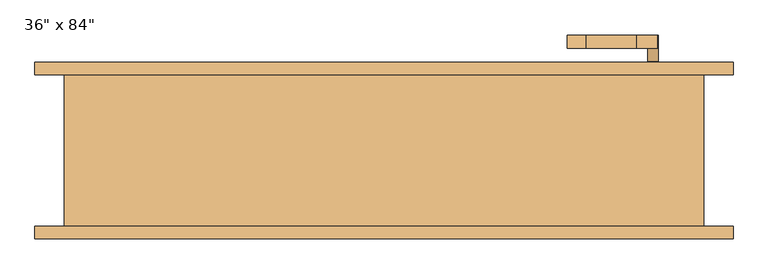
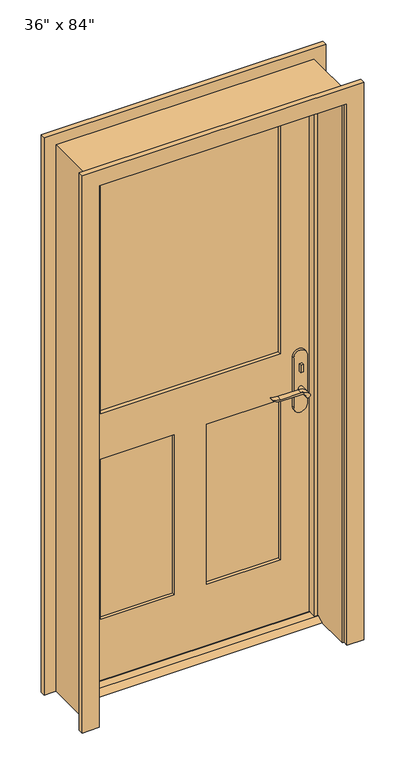
"""IFC4 building model written with IfcOpenShell, lengths in millimetres: door geometry."""

from ifc_helpers import new_model, si_unit, point, frame, frame_2d, origin, place, context, project, spatial, polyline, circle_curve, trimmed, segment, composite_curve, outline, extrude, faceted_brep, source, transform, mapped, element, save


def door_16625766(model_context):
    return source(origin(), model_context, "Body", "SolidModel", [
        extrude(outline(polyline([(38.1, 12.7), (73.025, 12.7), (98.425, 0.0), (12.7, 0.0), (38.1, 12.7)])), frame((-457.2, 0.0, 0.0), z_axis=(1.0, 0.0, 0.0), x_axis=(0.0, 1.0, 0.0)), (0.0, 0.0, 1.0), 914.4),
        extrude(outline(polyline([(411.4, 56.2), (401.4, 56.2), (401.4, 66.2), (411.4, 66.2), (411.4, 56.2)])), frame((0.0, 0.0, 981.9), z_axis=(0.0, 0.0, 1.0), x_axis=(1.0, 0.0, 0.0)), (0.0, 0.0, 1.0), 30.0),
        extrude(outline(composite_curve([segment(trimmed(circle_curve(frame_2d((996.9, 406.4)), 8.0), [point((996.9, 398.4))], [point((996.9, 414.4))], False, "CARTESIAN"), True, "CONTINUOUS"), segment(trimmed(circle_curve(frame_2d((996.9, 406.4)), 8.0), [point((996.9, 414.4))], [point((996.9, 398.4))], False, "CARTESIAN"), True, "CONTINUOUS")], self_intersect=False)), frame((0.0, 121.125, 0.0), z_axis=(0.0, 1.0, 0.0), x_axis=(0.0, 0.0, 1.0)), (0.0, 0.0, 1.0), 10.0),
        extrude(outline(composite_curve([segment(trimmed(circle_curve(frame_2d((897.1555521, 382.7324871)), 37.2832219), [point((919.0523287, 412.9081363))], [point((934.4, 381.0325667))], False, "CARTESIAN"), True, "CONTINUOUS"), segment(polyline([(934.4, 381.0325667), (934.4, 304.7564091)]), True, "CONTINUOUS"), segment(trimmed(circle_curve(frame_2d((1017.6850638, 304.8227909)), 83.2850902), [point((934.4, 304.7564091))], [point((939.4, 276.4))], True, "CARTESIAN"), True, "CONTINUOUS"), segment(polyline([(939.4, 276.4), (936.6135558, 276.4)]), True, "CONTINUOUS"), segment(trimmed(circle_curve(frame_2d((986.6709207, 308.3396612)), 59.3791355), [point((936.6135558, 276.4))], [point((927.4, 304.7564091))], False, "CARTESIAN"), True, "CONTINUOUS"), segment(polyline([(927.4, 304.7564091), (927.4, 381.0138099)]), True, "CONTINUOUS"), segment(trimmed(circle_curve(frame_2d((909.2738613, 381.0138099)), 18.1261387), [point((927.4, 381.0138099))], [point((914.4, 398.4))], True, "CARTESIAN"), True, "CONTINUOUS"), segment(trimmed(circle_curve(frame_2d((914.4, 406.4)), 8.0), [point((914.4, 398.4))], [point((919.0523287, 412.9081363))], False, "CARTESIAN"), True, "CONTINUOUS")], self_intersect=False)), frame((0.0, 16.2, 0.0), z_axis=(0.0, 1.0, 0.0), x_axis=(0.0, 0.0, 1.0)), (0.0, 0.0, 1.0), 20.0),
        extrude(outline(composite_curve([segment(trimmed(circle_curve(frame_2d((914.4, 406.4)), 8.0), [point((914.3999903, 398.4))], [point((919.0523287, 412.9081363))], False, "CARTESIAN"), True, "CONTINUOUS"), segment(trimmed(circle_curve(frame_2d((897.1555521, 382.7324871)), 37.2832219), [point((919.0523287, 412.9081363))], [point((934.4, 381.0325667))], False, "CARTESIAN"), True, "CONTINUOUS"), segment(polyline([(934.4, 381.0325667), (934.4, 304.7564091)]), True, "CONTINUOUS"), segment(trimmed(circle_curve(frame_2d((1017.6850638, 304.8227909)), 83.2850902), [point((934.4, 304.7564091))], [point((939.4, 276.4))], True, "CARTESIAN"), True, "CONTINUOUS"), segment(polyline([(939.4, 276.4), (936.6135558, 276.4)]), True, "CONTINUOUS"), segment(trimmed(circle_curve(frame_2d((986.6709207, 308.3396612)), 59.3791355), [point((936.6135558, 276.4))], [point((927.4, 304.7564091))], False, "CARTESIAN"), True, "CONTINUOUS"), segment(polyline([(927.4, 304.7564091), (927.4, 381.0138122)]), True, "CONTINUOUS"), segment(trimmed(circle_curve(frame_2d((909.2738682, 381.0138122)), 18.1261318), [point((927.4, 381.0138122))], [point((914.3999903, 398.4))], True, "CARTESIAN"), True, "CONTINUOUS")], self_intersect=False)), frame((0.0, 151.125, 0.0), z_axis=(0.0, 1.0, 0.0), x_axis=(0.0, 0.0, 1.0)), (0.0, 0.0, 1.0), 20.0),
        extrude(outline(composite_curve([segment(trimmed(circle_curve(frame_2d((914.4, 406.4)), 8.0), [point((914.4, 398.4))], [point((914.4, 414.4))], False, "CARTESIAN"), True, "CONTINUOUS"), segment(trimmed(circle_curve(frame_2d((914.4, 406.4)), 8.0), [point((914.4, 414.4))], [point((914.4, 398.4))], False, "CARTESIAN"), True, "CONTINUOUS")], self_intersect=False)), frame((0.0, 36.2, 0.0), z_axis=(0.0, 1.0, 0.0), x_axis=(0.0, 0.0, 1.0)), (0.0, 0.0, 1.0), 30.0),
        extrude(outline(composite_curve([segment(trimmed(circle_curve(frame_2d((914.4, 406.4)), 8.0), [point((914.4, 398.4))], [point((914.4, 414.4))], False, "CARTESIAN"), True, "CONTINUOUS"), segment(trimmed(circle_curve(frame_2d((914.4, 406.4)), 8.0), [point((914.4, 414.4))], [point((914.4, 398.4))], False, "CARTESIAN"), True, "CONTINUOUS")], self_intersect=False)), frame((0.0, 121.125, 0.0), z_axis=(0.0, 1.0, 0.0), x_axis=(0.0, 0.0, 1.0)), (0.0, 0.0, 1.0), 30.0),
        extrude(outline(composite_curve([segment(polyline([(844.4, 431.4), (1039.4, 431.4)]), True, "CONTINUOUS"), segment(trimmed(circle_curve(frame_2d((1039.4, 406.4)), 25.0), [point((1039.4, 431.4))], [point((1039.4, 381.4))], False, "CARTESIAN"), True, "CONTINUOUS"), segment(polyline([(1039.4, 381.4), (844.4, 381.4)]), True, "CONTINUOUS"), segment(trimmed(circle_curve(frame_2d((844.4, 406.4)), 25.0), [point((844.4, 381.4))], [point((844.4, 431.4))], False, "CARTESIAN"), True, "CONTINUOUS")], self_intersect=False)), frame((0.0, 66.2, 0.0), z_axis=(0.0, 1.0, 0.0), x_axis=(0.0, 0.0, 1.0)), (0.0, 0.0, 1.0), 10.0),
        extrude(outline(composite_curve([segment(polyline([(844.4, 431.4), (1039.4, 431.4)]), True, "CONTINUOUS"), segment(trimmed(circle_curve(frame_2d((1039.4, 406.4)), 25.0), [point((1039.4, 431.4))], [point((1039.4, 381.4))], False, "CARTESIAN"), True, "CONTINUOUS"), segment(polyline([(1039.4, 381.4), (844.4, 381.4)]), True, "CONTINUOUS"), segment(trimmed(circle_curve(frame_2d((844.4, 406.4)), 25.0), [point((844.4, 381.4))], [point((844.4, 431.4))], False, "CARTESIAN"), True, "CONTINUOUS")], self_intersect=False)), frame((0.0, 111.125, 0.0), z_axis=(0.0, 1.0, 0.0), x_axis=(0.0, 0.0, 1.0)), (0.0, 0.0, 1.0), 10.0),
        faceted_brep([(482.6, 111.125, 0.0), (482.6, -117.475, 0.0), (457.2, -117.475, 0.0), (457.2, 41.275, 0.0), (444.5, 41.275, 0.0), (444.5, 76.2, 0.0), (457.2, 76.2, 0.0), (457.2, 111.125, 0.0), (482.6, 111.125, 2159.0), (482.6, -117.475, 2159.0), (-482.6, -117.475, 2159.0), (-482.6, -117.475, 0.0), (-457.2, -117.475, 0.0), (-457.2, -117.475, 2133.6), (457.2, -117.475, 2133.6), (457.2, 41.275, 2133.6), (-457.2, 41.275, 2133.6), (-457.2, 41.275, 0.0), (-444.5, 41.275, 0.0), (-444.5, 41.275, 2120.9), (444.5, 41.275, 2120.9), (444.5, 76.2, 2120.9), (-444.5, 76.2, 2120.9), (-444.5, 76.2, 0.0), (-457.2, 76.2, 0.0), (-457.2, 76.2, 2133.6), (457.2, 76.2, 2133.6), (457.2, 111.125, 2133.6), (-457.2, 111.125, 2133.6), (-457.2, 111.125, 0.0), (-482.6, 111.125, 0.0), (-482.6, 111.125, 2159.0)], [[[0, 1, 2, 3, 4, 5, 6, 7]], [[1, 0, 8, 9]], [[2, 1, 9, 10, 11, 12, 13, 14]], [[3, 2, 14, 15]], [[4, 3, 15, 16, 17, 18, 19, 20]], [[5, 4, 20, 21]], [[6, 5, 21, 22, 23, 24, 25, 26]], [[7, 6, 26, 27]], [[0, 7, 27, 28, 29, 30, 31, 8]], [[9, 8, 31, 10]], [[15, 14, 13, 16]], [[21, 20, 19, 22]], [[27, 26, 25, 28]], [[30, 29, 24, 23, 18, 17, 12, 11]], [[10, 31, 30, 11]], [[16, 13, 12, 17]], [[22, 19, 18, 23]], [[28, 25, 24, 29]]]),
        extrude(outline(polyline([(2133.6, -457.2), (12.7, -457.2), (12.7, 457.2), (2133.6, 457.2), (2133.6, -457.2)]), holes=[polyline([(1066.8, -336.55), (2012.95, -336.55), (2012.95, 336.55), (1066.8, 336.55), (1066.8, -336.55)]), polyline([(885.825, -60.325), (254.0, -60.325), (254.0, -336.55), (885.825, -336.55), (885.825, -60.325)]), polyline([(885.825, 336.55), (254.0, 336.55), (254.0, 60.325), (885.825, 60.325), (885.825, 336.55)])]), frame((0.0, 76.2, 0.0), z_axis=(0.0, 1.0, 0.0), x_axis=(0.0, 0.0, 1.0)), (0.0, 0.0, 1.0), 34.925),
        extrude(outline(polyline([(336.55, 90.17), (-336.55, 90.17), (-336.55, 97.155), (336.55, 97.155), (336.55, 90.17)])), frame((0.0, 0.0, 1066.8), z_axis=(0.0, 0.0, 1.0), x_axis=(1.0, 0.0, 0.0)), (0.0, 0.0, 1.0), 946.15),
        extrude(outline(polyline([(-60.325, 87.8416667), (-336.55, 87.8416667), (-336.55, 99.4833333), (-60.325, 99.4833333), (-60.325, 87.8416667)])), frame((0.0, 0.0, 254.0), z_axis=(0.0, 0.0, 1.0), x_axis=(1.0, 0.0, 0.0)), (0.0, 0.0, 1.0), 631.825),
        extrude(outline(polyline([(336.55, 87.8416667), (60.325, 87.8416667), (60.325, 99.4833333), (336.55, 99.4833333), (336.55, 87.8416667)])), frame((0.0, 0.0, 254.0), z_axis=(0.0, 0.0, 1.0), x_axis=(1.0, 0.0, 0.0)), (0.0, 0.0, 1.0), 631.825),
        extrude(outline(polyline([(0.0, -527.05), (0.0, -463.55), (2139.95, -463.55), (2139.95, 463.55), (0.0, 463.55), (0.0, 527.05), (2203.45, 527.05), (2203.45, -527.05), (0.0, -527.05)])), frame((0.0, 111.125, 0.0), z_axis=(0.0, 1.0, 0.0), x_axis=(0.0, 0.0, 1.0)), (0.0, 0.0, 1.0), 19.05),
        extrude(outline(polyline([(0.0, -527.05), (0.0, -463.55), (2139.95, -463.55), (2139.95, 463.55), (0.0, 463.55), (0.0, 527.05), (2203.45, 527.05), (2203.45, -527.05), (0.0, -527.05)])), frame((0.0, -136.525, 0.0), z_axis=(0.0, 1.0, 0.0), x_axis=(0.0, 0.0, 1.0)), (0.0, 0.0, 1.0), 19.05),
    ])


if __name__ == "__main__":
    model = new_model("IFC4")
    model_context = context("Model", 3, world=origin())
    ifc_project = project(units=[si_unit("LENGTHUNIT", "METRE", prefix="MILLI")], contexts=[model_context])
    site = spatial("IfcSite", under=ifc_project)
    building = spatial("IfcBuilding", under=site)
    placement = place(None, origin())
    door_shape = door_16625766(model_context)
    element("IfcDoor", 1, ObjectType="36\" x 84\"", at=placement, inside=building, context=model_context, shape_type="MappedRepresentation", body=[
        mapped(door_shape, transform((0.0, 0.0, 0.0), x_axis=(1.0, 0.0, 0.0), y_axis=(0.0, 1.0, 0.0), z_axis=(0.0, 0.0, 1.0))),
    ])
    save(model, "model.ifc")

# Revit data of these elements
# Type "36\" x 84\""
#   Type Mark = "8"
#   Assembly Code = "B2030100"
#   Analytic Construction = "French door, wood frame with single glass"
#   Top Rail = 0' - 4 3/4"
#   Threshold Offset [instance default] = 0' - 0 1/2"
#   Thickness = 0' - 1 3/8"
#   Thermal Resistance (R) = 1.0696 (h·ft²·°F)/BTU
#   Swing Angle [instance default] = 90.00°
#   Stiles = 0' - 4 3/4"
#   Rough Width = 3' - 2"
#   Rough Height = 7' - 1"
#   Lock Rail = 0' - 7 1/8"
#   Height = 7' - 0"
#   Width = 3' - 0"
#   Heat Transfer Coefficient (U) = 0.9350 BTU/(h·ft²·°F)
#   Door Offset [instance default] = 0' - 0"
#   Bottom Rail = 0' - 9 1/2"
#   Threshold [instance default] = yes
#   Function = 1
#   Exterior Trim [instance default] = yes
#   Trim Material = Cherry
#   Threshold Material = Cherry
#   Panel Material = Cherry
#   Glazing = Glass
#   Frame Material = Cherry
#   Door Handle Material = Aluminum
#   Visual Light Transmittance = 0
#   Solar Heat Gain Coefficient = 0
#   Wall Closure = (empty or 0)
#   Construction Type = (empty or 0)
# Element 1 (IfcDoor, "36\" x 84\"")
#   Materials on its faces: "Cherry", "Aluminum", "Glass"
# Materials
#   "Cherry": class "Wood", colour RGB 226 177 128, transparency 0, Description = "Prunus Serotina", Cost = 0
#   "Glass": class "Glass", colour RGB 0 128 192, transparency 0.75, Description = "Soda Lime Glass", Cost = 0
#   "Aluminum": class "Metal", colour RGB 247 247 247, transparency 0, Description = "Aluminum 6061", Cost = 0
